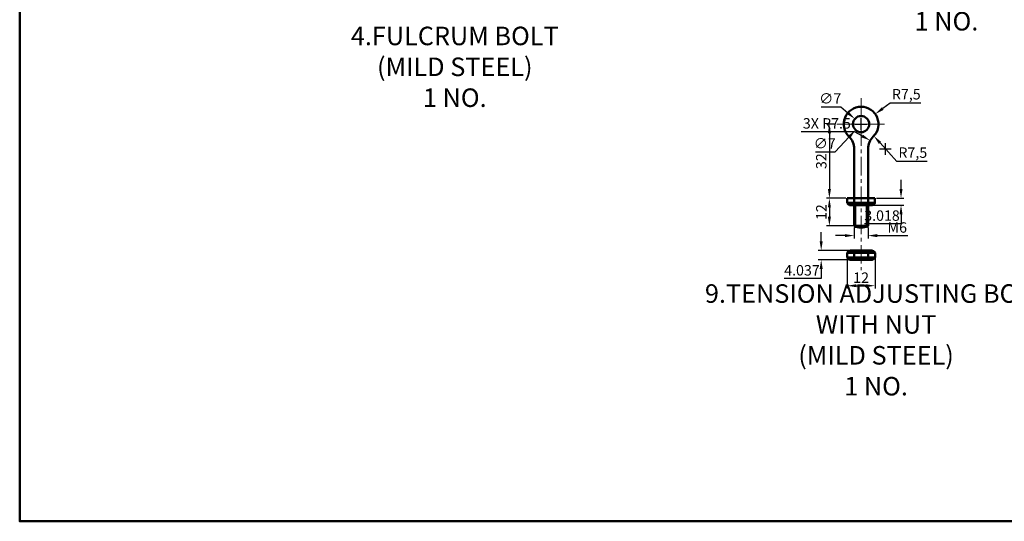
# Model space of a CAD drawing. Units: millimetres. Extents: x -166 to 681, y -4360 to 126.
# Tile 1 of 7: x -166 to 259, y -430 to -213. Entities that reach past the tile are written whole.
import ezdxf

# ---------------------------------------------------------------- set-up
doc = ezdxf.new("R2010")
doc.units = ezdxf.units.MM
doc.header["$LTSCALE"] = 0.5
doc.linetypes.add('CENTER', pattern=[50.8, 31.75, -6.35, 6.35, -6.35])
for name, color, linetype, lineweight in [('M-CNTR', 1, 'CENTER', 18), ('M-DIMS', 2, 'Continuous', 25), ('M-OUTL', 7, 'Continuous', 50), ('M-TEXT', 7, 'Continuous', 25), ('M-TTLB', 7, 'Continuous', 50)]:
    doc.layers.add(name, color=color, linetype=linetype, lineweight=lineweight)
doc.styles.get("Standard").update_dxf_attribs({"font": 'arial.ttf'})
doc.dimstyles.new('ISO-25', dxfattribs={"dimtxt": 4.5, "dimasz": 4, "dimexe": 1.25, "dimexo": 0.625, "dimtad": 1, "dimtoh": 1, "dimdec": 1, "dimtxsty": 'Standard', "dimcen": 2.5, "dimadec": 0, "dimazin": 0, "dimtfac": 1, "dimtdec": 1, "dimtofl": 0, "dimtmove": 0, "dimatfit": 3, "dimfxl": 1, "dimarcsym": 0})

# ---------------------------------------------------------------- blocks, each defined once
blk = doc.blocks.new('*D57')
at = {"layer": 'Defpoints', "color": 0, "ltscale": 0.5, "transparency": 16777216}
for p in [(186.76, -258.45), (183.6, -290.45), (191.29, -290.45)]:
    blk.add_point(p, dxfattribs=at)
at = {"layer": 'M-DIMS', "color": 0, "lineweight": -2, "ltscale": 0.5, "transparency": 16777216}
for p, q in [((186.14, -258.45), (182.35, -258.45)), ((183.6, -262.45), (183.6, -286.45)), ((190.66, -290.45), (182.35, -290.45))]:
    blk.add_line(p, q, dxfattribs=at)
at = {"layer": 'M-DIMS', "color": 0, "ltscale": 0.5, "transparency": 16777216}
for points in [[(182.94, -262.45), (184.27, -262.45), (183.6, -258.45)], [(182.94, -286.45), (184.27, -286.45), (183.6, -290.45)]]:
    blk.add_solid(points, dxfattribs=at)
at = {"layer": 'M-DIMS', "color": 0, "ltscale": 0.5, "transparency": 16777216, "insert": (180.68, -274.45), "char_height": 4.5, "attachment_point": 5, "rotation": 90}
blk.add_mtext('32', dxfattribs=at)
blk = doc.blocks.new('*D58')
at = {"layer": 'Defpoints', "color": 0, "ltscale": 0.5, "transparency": 16777216}
for p in [(191.29, -290.45), (183.6, -302.45), (194.29, -302.45)]:
    blk.add_point(p, dxfattribs=at)
at = {"layer": 'M-DIMS', "color": 0, "lineweight": -2, "ltscale": 0.5, "transparency": 16777216}
for p, q in [((190.66, -290.45), (182.35, -290.45)), ((183.6, -294.45), (183.6, -298.45)), ((193.66, -302.45), (182.35, -302.45))]:
    blk.add_line(p, q, dxfattribs=at)
at = {"layer": 'M-DIMS', "color": 0, "ltscale": 0.5, "transparency": 16777216}
for points in [[(182.94, -294.45), (184.27, -294.45), (183.6, -290.45)], [(182.94, -298.45), (184.27, -298.45), (183.6, -302.45)]]:
    blk.add_solid(points, dxfattribs=at)
at = {"layer": 'M-DIMS', "color": 0, "ltscale": 0.5, "transparency": 16777216, "insert": (180.72, -296.45), "char_height": 4.5, "attachment_point": 5, "rotation": 90}
blk.add_mtext('12', dxfattribs=at)
blk = doc.blocks.new('*D59')
at = {"layer": 'Defpoints', "color": 0, "ltscale": 0.5, "transparency": 16777216}
for p in [(194.29, -302.45), (200.29, -302.45), (200.29, -306.6)]:
    blk.add_point(p, dxfattribs=at)
at = {"layer": 'M-DIMS', "color": 0, "lineweight": -2, "ltscale": 0.5, "transparency": 16777216}
for p, q in [((194.29, -303.07), (194.29, -307.85)), ((200.29, -303.07), (200.29, -307.85)), ((190.29, -306.6), (186.29, -306.6)), ((204.29, -306.6), (217.52, -306.6))]:
    blk.add_line(p, q, dxfattribs=at)
at = {"layer": 'M-DIMS', "color": 0, "ltscale": 0.5, "transparency": 16777216}
for points in [[(190.29, -305.94), (190.29, -307.27), (194.29, -306.6)], [(204.29, -305.94), (204.29, -307.27), (200.29, -306.6)]]:
    blk.add_solid(points, dxfattribs=at)
at = {"layer": 'M-DIMS', "color": 0, "ltscale": 0.5, "transparency": 16777216, "insert": (212.9, -303.68), "char_height": 4.5, "attachment_point": 5}
blk.add_mtext('M6', dxfattribs=at)
blk = doc.blocks.new('*D60')
at = {"layer": 'Defpoints', "color": 0, "ltscale": 0.5, "transparency": 16777216}
for p in [(202.78, -263.57), (207.79, -269.16)]:
    blk.add_point(p, dxfattribs=at)
at = {"layer": 'M-DIMS', "color": 0, "lineweight": -2, "ltscale": 0.5, "transparency": 16777216}
for p, q in [((212.72, -274.66), (205.45, -266.55)), ((225.88, -274.66), (212.72, -274.66))]:
    blk.add_line(p, q, dxfattribs=at)
blk.add_arc((207.79, -269.16), 7.5, 122.3328, 134.427, dxfattribs=at)
at = {"layer": 'M-DIMS', "color": 0, "ltscale": 0.5, "transparency": 16777216}
blk.add_solid([(205.95, -266.11), (204.96, -267), (202.78, -263.57)], dxfattribs=at)
at = {"layer": 'M-DIMS', "color": 0, "ltscale": 0.5, "transparency": 16777216, "insert": (219.61, -271.34), "char_height": 4.5, "attachment_point": 5}
blk.add_mtext('R7,5', dxfattribs=at)
blk = doc.blocks.new('*D61')
at = {"layer": 'Defpoints', "color": 0, "ltscale": 0.5, "transparency": 16777216}
for p in [(203.4, -254.09), (197.29, -258.45)]:
    blk.add_point(p, dxfattribs=at)
at = {"layer": 'M-DIMS', "color": 0, "lineweight": -2, "ltscale": 0.5, "transparency": 16777216}
for p, q in [((209.91, -249.45), (206.65, -251.77)), ((223.07, -249.45), (209.91, -249.45)), ((194.79, -258.45), (199.79, -258.45)), ((197.29, -260.95), (197.29, -255.95))]:
    blk.add_line(p, q, dxfattribs=at)
at = {"layer": 'M-DIMS', "color": 0, "ltscale": 0.5, "transparency": 16777216}
blk.add_solid([(206.27, -251.23), (207.04, -252.31), (203.4, -254.09)], dxfattribs=at)
at = {"layer": 'M-DIMS', "color": 0, "ltscale": 0.5, "transparency": 16777216, "insert": (216.8, -246.13), "char_height": 4.5, "attachment_point": 5}
blk.add_mtext('R7,5', dxfattribs=at)
blk = doc.blocks.new('*D62')
at = {"layer": 'Defpoints', "color": 0, "ltscale": 0.5, "transparency": 16777216}
for p in [(194.61, -256.19), (199.96, -260.7)]:
    blk.add_point(p, dxfattribs=at)
at = {"layer": 'M-DIMS', "color": 0, "lineweight": -2, "ltscale": 0.5, "transparency": 16777216}
for p, q in [((180.03, -251.03), (188.5, -251.03)), ((188.5, -251.03), (191.56, -253.61)), ((194.79, -258.45), (199.79, -258.45)), ((197.29, -260.95), (197.29, -255.95))]:
    blk.add_line(p, q, dxfattribs=at)
at = {"layer": 'M-DIMS', "color": 0, "ltscale": 0.5, "transparency": 16777216}
blk.add_solid([(191.99, -253.1), (191.13, -254.12), (194.61, -256.19)], dxfattribs=at)
at = {"layer": 'M-DIMS', "color": 0, "ltscale": 0.5, "transparency": 16777216, "insert": (183.95, -247.98), "char_height": 4.5, "attachment_point": 5}
blk.add_mtext('∅7', dxfattribs=at)
blk = doc.blocks.new('*D89')
at = {"layer": 'Defpoints', "color": 0, "ltscale": 0.5, "transparency": 16777216}
for p in [(191.3, -314.07), (203.3, -314.07), (203.3, -328.25)]:
    blk.add_point(p, dxfattribs=at)
at = {"layer": 'M-DIMS', "color": 0, "lineweight": -2, "ltscale": 0.5, "transparency": 16777216}
for p, q in [((191.3, -314.7), (191.3, -329.5)), ((203.3, -314.7), (203.3, -329.5)), ((195.3, -328.25), (199.3, -328.25))]:
    blk.add_line(p, q, dxfattribs=at)
at = {"layer": 'M-DIMS', "color": 0, "ltscale": 0.5, "transparency": 16777216}
for points in [[(195.3, -327.58), (195.3, -328.91), (191.3, -328.25)], [(199.3, -327.58), (199.3, -328.91), (203.3, -328.25)]]:
    blk.add_solid(points, dxfattribs=at)
at = {"layer": 'M-DIMS', "color": 0, "ltscale": 0.5, "transparency": 16777216, "insert": (197.3, -325.36), "char_height": 4.5, "attachment_point": 5}
blk.add_mtext('12', dxfattribs=at)
blk = doc.blocks.new('*D90')
at = {"layer": 'Defpoints', "color": 0, "ltscale": 0.5, "transparency": 16777216}
for p in [(203.29, -290.45), (201.79, -293.46), (214.53, -293.46)]:
    blk.add_point(p, dxfattribs=at)
at = {"layer": 'M-DIMS', "color": 0, "lineweight": -2, "ltscale": 0.5, "transparency": 16777216}
for p, q in [((214.53, -286.45), (214.53, -282.45)), ((203.91, -290.45), (215.78, -290.45)), ((202.41, -293.46), (215.78, -293.46)), ((214.53, -297.46), (214.53, -301.46)), ((214.53, -301.46), (198.72, -301.46))]:
    blk.add_line(p, q, dxfattribs=at)
at = {"layer": 'M-DIMS', "color": 0, "ltscale": 0.5, "transparency": 16777216}
for points in [[(213.87, -286.45), (215.2, -286.45), (214.53, -290.45)], [(213.87, -297.46), (215.2, -297.46), (214.53, -293.46)]]:
    blk.add_solid(points, dxfattribs=at)
at = {"layer": 'M-DIMS', "color": 0, "ltscale": 0.5, "transparency": 16777216, "insert": (206.31, -298.54), "char_height": 4.5, "attachment_point": 5}
blk.add_mtext('3.018', dxfattribs=at)
blk = doc.blocks.new('*D91')
at = {"layer": 'Defpoints', "color": 0, "ltscale": 0.5, "transparency": 16777216}
for p in [(192.8, -313.06), (180.06, -317.09), (192.8, -317.09)]:
    blk.add_point(p, dxfattribs=at)
at = {"layer": 'M-DIMS', "color": 0, "lineweight": -2, "ltscale": 0.5, "transparency": 16777216}
for p, q in [((180.06, -309.06), (180.06, -305.06)), ((192.18, -313.06), (178.81, -313.06)), ((192.18, -317.09), (178.81, -317.09)), ((180.06, -321.09), (180.06, -325.09)), ((180.06, -325.09), (164.07, -325.09))]:
    blk.add_line(p, q, dxfattribs=at)
at = {"layer": 'M-DIMS', "color": 0, "ltscale": 0.5, "transparency": 16777216}
for points in [[(179.4, -309.06), (180.73, -309.06), (180.06, -313.06)], [(179.4, -321.09), (180.73, -321.09), (180.06, -317.09)]]:
    blk.add_solid(points, dxfattribs=at)
at = {"layer": 'M-DIMS', "color": 0, "ltscale": 0.5, "transparency": 16777216, "insert": (171.76, -322.17), "char_height": 4.5, "attachment_point": 5}
blk.add_mtext('4.037', dxfattribs=at)
blk = doc.blocks.new('*D104')
at = {"layer": 'Defpoints', "color": 0, "ltscale": 0.5, "transparency": 16777216}
for p in [(199.68, -255.89), (194.9, -261.01)]:
    blk.add_point(p, dxfattribs=at)
at = {"layer": 'M-DIMS', "color": 0, "lineweight": -2, "ltscale": 0.5, "transparency": 16777216}
for p, q in [((194.79, -258.45), (199.79, -258.45)), ((197.29, -260.95), (197.29, -255.95)), ((186.14, -270.4), (192.17, -263.93)), ((177.67, -270.4), (186.14, -270.4))]:
    blk.add_line(p, q, dxfattribs=at)
at = {"layer": 'M-DIMS', "color": 0, "ltscale": 0.5, "transparency": 16777216}
blk.add_solid([(191.69, -263.48), (192.66, -264.39), (194.9, -261.01)], dxfattribs=at)
at = {"layer": 'M-DIMS', "color": 0, "ltscale": 0.5, "transparency": 16777216, "insert": (181.59, -267.35), "char_height": 4.5, "attachment_point": 5}
blk.add_mtext('∅7', dxfattribs=at)
blk = doc.blocks.new('*D105')
at = {"layer": 'Defpoints', "color": 0, "ltscale": 0.5, "transparency": 16777216}
for p in [(201.23, -265.52), (207.79, -269.16)]:
    blk.add_point(p, dxfattribs=at)
at = {"layer": 'M-DIMS', "color": 0, "lineweight": -2, "ltscale": 0.5, "transparency": 16777216}
for p, q in [((171.41, -261.63), (194.24, -261.63)), ((194.24, -261.63), (197.73, -263.58)), ((207.79, -271.66), (207.79, -266.66)), ((205.29, -269.16), (210.29, -269.16))]:
    blk.add_line(p, q, dxfattribs=at)
at = {"layer": 'M-DIMS', "color": 0, "ltscale": 0.5, "transparency": 16777216}
blk.add_solid([(198.06, -262.99), (197.41, -264.16), (201.23, -265.52)], dxfattribs=at)
at = {"layer": 'M-DIMS', "color": 0, "ltscale": 0.5, "transparency": 16777216, "insert": (182.51, -258.71), "char_height": 4.5, "attachment_point": 5}
blk.add_mtext('3X R7.5', dxfattribs=at)

msp = doc.modelspace()

# ---------------------------------------------------------------- linework, layer by layer
at = {"layer": 'M-CNTR', "ltscale": 0.5}
for p, q in [((197.2887, -247.245), (197.2887, -321.5483)), ((186.7646, -258.4454), (207.8342, -258.4454))]:
    msp.add_line(p, q, dxfattribs=at)
at = {"layer": 'M-OUTL', "ltscale": 0.5}
for p, q in [((194.2887, -269.1575), (194.2887, -302.4454)), ((200.2887, -269.1575), (200.2887, -302.4454)), ((191.2887, -292.4454), (191.2887, -290.4454)), ((191.2887, -290.4454), (203.2887, -290.4454)), ((203.2887, -292.4454), (191.2887, -292.4454)), ((203.2887, -290.4454), (203.2887, -292.4454)), ((202.0289, -293.4454), (192.5715, -293.4454)), ((194.2887, -293.4454), (194.2887, -302.4454)), ((194.7887, -293.4454), (194.7887, -302.4454)), ((199.7887, -293.4454), (199.7887, -302.4454)), ((194.2887, -302.4454), (200.2887, -302.4454)), ((191.3002, -314.0748), (203.3002, -314.0748)), ((191.3002, -314.0748), (191.3002, -316.076)), ((192.56, -313.0748), (202.0174, -313.0748)), ((194.3002, -314.0748), (194.3037, -316.076)), ((200.3002, -314.0748), (200.3037, -316.076)), ((203.3002, -314.0748), (203.3037, -316.076)), ((191.3037, -316.076), (203.3037, -316.076)), ((192.5635, -317.076), (202.0209, -317.076))]:
    msp.add_line(p, q, dxfattribs=at)
msp.add_circle((197.2887, -258.4454), 3.5, dxfattribs=at)
for centre, radius, start, end in [((197.2887, -258.4454), 7.5, 314.427004, 225.572996), ((186.7887, -269.1575), 7.5, 0, 45.572996), ((207.7887, -269.1575), 7.5, 134.427004, 180), ((192.7887, -291.844), 1.6161, 201.847759, 338.152241), ((197.2887, -288.4454), 5, 233.130102, 306.869898), ((201.7887, -291.8492), 1.6141, 201.6745, 338.3255), ((197.2887, -296.6121), 6.5595, 242.783818, 297.216182), ((192.8002, -314.6709), 1.6141, 21.6745, 158.3255), ((197.3002, -318.0748), 5, 53.130102, 126.869898), ((201.8002, -314.6762), 1.6161, 21.847759, 158.152241), ((192.8037, -315.4799), 1.6141, 201.6745, 338.3255), ((197.3037, -312.076), 5, 233.130102, 306.869898), ((201.8037, -315.4746), 1.6161, 201.847759, 338.152241)]:
    msp.add_arc(centre, radius, start, end, dxfattribs=at)
at = {"layer": 'M-TTLB', "ltscale": 0.5}
msp.add_lwpolyline([(-165.9437, 126.0872), (680.7907, 126.0872), (680.7907, -430.0081), (-165.9437, -430.0081)], close=True, dxfattribs=at)

# ---------------------------------------------------------------- texts
at = {"layer": 'M-TEXT', "ltscale": 0.5, "char_height": 8, "attachment_point": 1}
for s, insert in [('\\pxqc;6.STEM (MILD STEEL) \\P1 NO.', (158.6774, -196.6773)), ('\\pxqc;4.FULCRUM BOLT\\P(MILD STEEL) \\P1 NO.', (-53.5871, -216.3668)), ('\\pxqc;9.TENSION ADJUSTING BOLT WITH NUT\\P(MILD STEEL) \\P1 NO.', (128.2808, -327.6326))]:
    msp.add_mtext_dynamic_manual_height_columns(s, width=150.92987, gutter_width=12.5, heights=[0], dxfattribs=dict(at, insert=insert))

# ---------------------------------------------------------------- dimensions: what is measured, and where the dimension line sits
at = {"layer": 'M-DIMS', "ltscale": 0.5}
dim = msp.add_diameter_dim_2p(p1=(199.9637, -260.7025), p2=(194.6137, -256.1883), dimstyle='ISO-25', override={"dimclrd": 0, "dimclre": 0, "dimclrt": 0}, dxfattribs=at)
dim.commit()
dim.dimension.update_dxf_attribs({"geometry": '*D62', "text_midpoint": (183.9515, -247.9809)})
dim = msp.add_radius_dim(center=(197.2887, -258.4454), mpoint=(203.3962, -254.0924), dimstyle='ISO-25', override={"dimclrd": 0, "dimclre": 0, "dimclrt": 0}, dxfattribs=at)
dim.commit()
dim.dimension.update_dxf_attribs({"geometry": '*D61', "text_midpoint": (216.8024, -246.1292)})
dim = msp.add_radius_dim(center=(207.7887, -269.1575), mpoint=(201.2313, -265.5174), text='3X <>', dimstyle='ISO-25', override={"dimdec": 1, "dimlfac": 1, "dimrnd": 0, "dimzin": 0, "dimdsep": 46, "dimlunit": 2}, dxfattribs=at)
dim.commit()
dim.dimension.update_dxf_attribs({"geometry": '*D105', "text_midpoint": (182.5122, -258.7104)})
dim = msp.add_diameter_dim_2p(p1=(199.6755, -255.8855), p2=(194.9018, -261.0053), dimstyle='ISO-25', override={"dimdec": 0, "dimlfac": 1, "dimrnd": 0, "dimzin": 0, "dimdsep": 46, "dimlunit": 2}, dxfattribs=at)
dim.commit()
dim.dimension.update_dxf_attribs({"geometry": '*D104', "text_midpoint": (181.5929, -270.4014), "dimtype": 163})
for base, p1, p2, override, picture, middle in [((183.6045, -290.4454), (186.7646, -258.4454), (191.2887, -290.4454), {"dimclrd": 0, "dimclre": 0, "dimclrt": 0}, '*D57', (180.6803, -274.4454)), ((214.5342, -293.4634), (203.2887, -290.4454), (201.7887, -293.4634), {"dimdec": 3, "dimlfac": 1, "dimrnd": 0, "dimzin": 0, "dimdsep": 46, "dimlunit": 2}, '*D90', (206.3136, -298.5393)), ((183.6045, -302.4454), (191.2887, -290.4454), (194.2887, -302.4454), {"dimclrd": 0, "dimclre": 0, "dimclrt": 0}, '*D58', (180.7203, -296.4454)), ((180.0646, -317.094), (192.8002, -313.0568), (192.8037, -317.094), {"dimdec": 3, "dimlfac": 1, "dimrnd": 0, "dimzin": 0, "dimdsep": 46, "dimlunit": 2}, '*D91', (171.7564, -322.1699))]:
    dim = msp.add_linear_dim(base=base, p1=p1, p2=p2, angle=90, dimstyle='ISO-25', override=override, dxfattribs=at)
    dim.commit()
    dim.dimension.update_dxf_attribs({"geometry": picture, "text_midpoint": middle})
dim = msp.add_radius_dim(center=(207.7887, -269.1575), mpoint=(202.7817, -263.5736), dimstyle='ISO-25', override={"dimclrd": 0, "dimclre": 0, "dimclrt": 0}, dxfattribs=at)
dim.commit()
dim.dimension.update_dxf_attribs({"geometry": '*D60', "text_midpoint": (219.6148, -274.6607), "dimtype": 164})
dim = msp.add_linear_dim(base=(200.2887, -306.605), p1=(194.2887, -302.4454), p2=(200.2887, -302.4454), text='M<>', dimstyle='ISO-25', override={"dimclrd": 0, "dimclre": 0, "dimclrt": 0}, dxfattribs=at)
dim.commit()
dim.dimension.update_dxf_attribs({"geometry": '*D59', "text_midpoint": (212.9026, -306.605), "dimtype": 160})
dim = msp.add_linear_dim(base=(203.3002, -328.2483), p1=(191.3002, -314.0748), p2=(203.3002, -314.0748), dimstyle='ISO-25', override={"dimdec": 0, "dimlfac": 1, "dimrnd": 0, "dimzin": 0, "dimdsep": 46, "dimlunit": 2}, dxfattribs=at)
dim.commit()
dim.dimension.update_dxf_attribs({"geometry": '*D89', "text_midpoint": (197.3002, -325.3641)})

doc.saveas('drawing.dxf')
